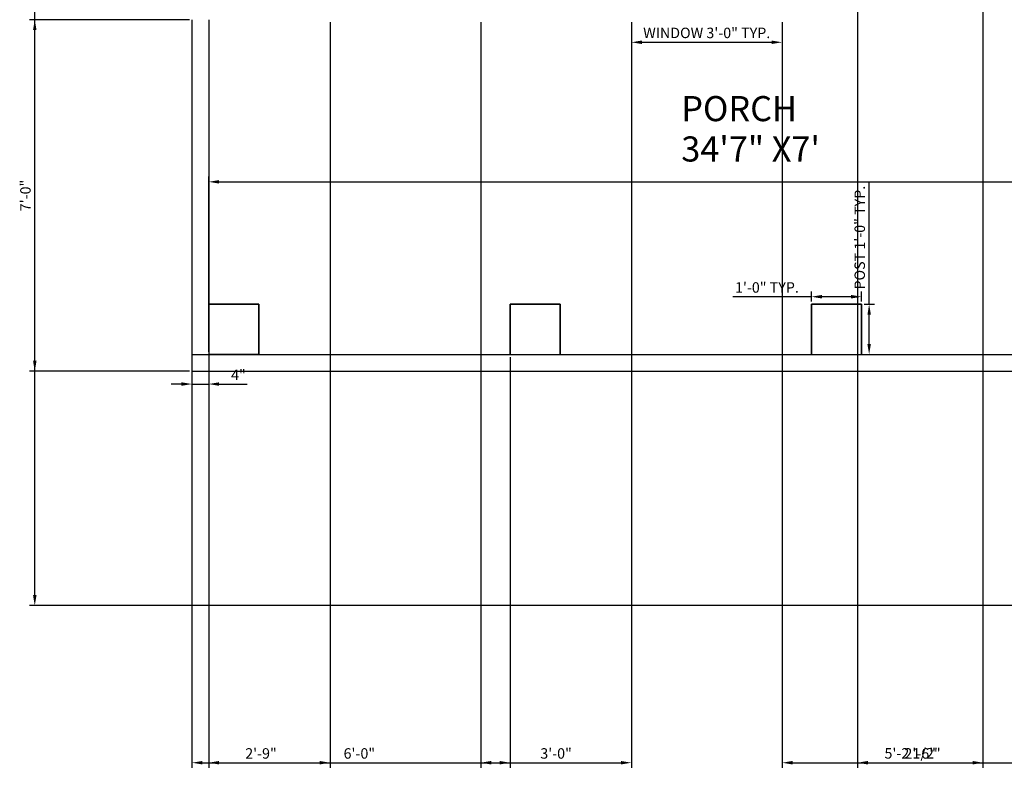
# Model space of a CAD drawing. Units: inches. Extents: x 2025 to 2528, y 1525 to 2336.
# Tile 1 of 18: x 2025 to 2260, y 1525 to 1704. Entities that reach past the tile are written whole.
import ezdxf

# ---------------------------------------------------------------- set-up
doc = ezdxf.new("R2010")
doc.units = ezdxf.units.IN
for name, color, linetype, lineweight in [('A-ANNO-DIMS', 2, 'Continuous', 18), ('A-AREA-IDEN', 7, 'Continuous', 25), ('A-COLS', 7, 'Continuous', 35), ('A-FLOR', 7, 'Continuous', 25)]:
    doc.layers.add(name, color=color, linetype=linetype, lineweight=lineweight)
doc.styles.get("Standard").update_dxf_attribs({"font": 'arial.ttf'})
doc.dimstyles.new('Copy of ISO-25', dxfattribs={"dimtxt": 2.5, "dimasz": 2.5, "dimexe": 1.25, "dimexo": 0.625, "dimtad": 1, "dimdec": 1, "dimlunit": 4, "dimtxsty": 'Standard', "dimcen": 2.5, "dimadec": 0, "dimazin": 0, "dimtfac": 1, "dimtdec": 1, "dimtmove": 0, "dimatfit": 3, "dimfxl": 1, "dimarcsym": 0})

# ---------------------------------------------------------------- blocks, each defined once
blk = doc.blocks.new('*D40')
at = {"layer": 'A-ANNO-DIMS', "color": 0, "lineweight": -2, "transparency": 16777216}
for p, q in [((2070.01, 1625.04), (2070.01, 1666.92)), ((2072.51, 1665.67), (2482.51, 1665.67)), ((2485.01, 1625.04), (2485.01, 1666.92))]:
    blk.add_line(p, q, dxfattribs=at)
at = {"layer": 'A-ANNO-DIMS', "color": 0, "transparency": 16777216}
for points in [[(2072.51, 1666.08), (2072.51, 1665.25), (2070.01, 1665.67)], [(2482.51, 1666.08), (2482.51, 1665.25), (2485.01, 1665.67)]]:
    blk.add_solid(points, dxfattribs=at)
at = {"layer": 'Defpoints', "color": 0, "transparency": 16777216}
for p in [(2485.01, 1665.67), (2070.01, 1624.41), (2485.01, 1624.41)]:
    blk.add_point(p, dxfattribs=at)
at = {"layer": 'A-ANNO-DIMS', "color": 0, "transparency": 16777216, "insert": (2277.51, 1667.57), "char_height": 2.5, "attachment_point": 5}
blk.add_mtext('34\'-7"', dxfattribs=at)
blk = doc.blocks.new('*D44')
at = {"layer": 'A-ANNO-DIMS', "color": 0, "lineweight": -2, "transparency": 16777216}
for p, q in [((2066.01, 1619.79), (2066.01, 1616.1)), ((2070.01, 1619.79), (2070.01, 1616.1)), ((2063.51, 1617.35), (2061.01, 1617.35)), ((2066.01, 1617.35), (2070.01, 1617.35)), ((2072.51, 1617.35), (2079.24, 1617.35))]:
    blk.add_line(p, q, dxfattribs=at)
at = {"layer": 'A-ANNO-DIMS', "color": 0, "transparency": 16777216}
for points in [[(2063.51, 1617.76), (2063.51, 1616.93), (2066.01, 1617.35)], [(2072.51, 1617.76), (2072.51, 1616.93), (2070.01, 1617.35)]]:
    blk.add_solid(points, dxfattribs=at)
at = {"layer": 'Defpoints', "color": 0, "transparency": 16777216}
for p in [(2066.01, 1620.41), (2070.01, 1620.41), (2070.01, 1617.35)]:
    blk.add_point(p, dxfattribs=at)
at = {"layer": 'A-ANNO-DIMS', "color": 0, "transparency": 16777216, "insert": (2077.12, 1619.22), "char_height": 2.5, "attachment_point": 5}
blk.add_mtext('4"', dxfattribs=at)
blk = doc.blocks.new('POST-PORCH-12')
for p, q in [((12, 12), (0, 12)), ((12, 0), (12, 12)), ((0, 0), (12, 0))]:
    blk.add_line(p, q)
blk = doc.blocks.new('*D50')
at = {"layer": 'A-ANNO-DIMS', "color": 0, "lineweight": -2, "transparency": 16777216}
for p, q in [((2227.81, 1636.41), (2227.81, 1665.76)), ((2226.64, 1636.41), (2229.06, 1636.41)), ((2227.81, 1626.91), (2227.81, 1633.91)), ((2226.64, 1624.41), (2229.06, 1624.41))]:
    blk.add_line(p, q, dxfattribs=at)
at = {"layer": 'A-ANNO-DIMS', "color": 0, "transparency": 16777216}
for points in [[(2227.4, 1633.91), (2228.23, 1633.91), (2227.81, 1636.41)], [(2227.4, 1626.91), (2228.23, 1626.91), (2227.81, 1624.41)]]:
    blk.add_solid(points, dxfattribs=at)
at = {"layer": 'Defpoints', "color": 0, "transparency": 16777216}
for p in [(2226.01, 1636.41), (2227.81, 1636.41), (2226.01, 1624.41)]:
    blk.add_point(p, dxfattribs=at)
at = {"layer": 'A-ANNO-DIMS', "color": 0, "transparency": 16777216, "insert": (2225.89, 1652.33), "char_height": 2.5, "attachment_point": 5, "rotation": 90}
blk.add_mtext('POST 1\'-0" TYP.', dxfattribs=at)
blk = doc.blocks.new('*D51')
at = {"layer": 'A-ANNO-DIMS', "color": 0, "lineweight": -2, "transparency": 16777216}
for p, q in [((2214.01, 1638.21), (2195.26, 1638.21)), ((2214.01, 1637.04), (2214.01, 1639.46)), ((2223.51, 1638.21), (2216.51, 1638.21)), ((2226.01, 1637.04), (2226.01, 1639.46))]:
    blk.add_line(p, q, dxfattribs=at)
at = {"layer": 'A-ANNO-DIMS', "color": 0, "transparency": 16777216}
for points in [[(2216.51, 1638.63), (2216.51, 1637.8), (2214.01, 1638.21)], [(2223.51, 1638.63), (2223.51, 1637.8), (2226.01, 1638.21)]]:
    blk.add_solid(points, dxfattribs=at)
at = {"layer": 'Defpoints', "color": 0, "transparency": 16777216}
for p in [(2214.01, 1638.21), (2214.01, 1636.41), (2226.01, 1636.41)]:
    blk.add_point(p, dxfattribs=at)
at = {"layer": 'A-ANNO-DIMS', "color": 0, "transparency": 16777216, "insert": (2203.39, 1640.11), "char_height": 2.5, "attachment_point": 5}
blk.add_mtext('1\'-0" TYP.', dxfattribs=at)
blk = doc.blocks.new('*D52')
at = {"layer": 'A-ANNO-DIMS', "color": 0, "lineweight": -2, "transparency": 16777216}
for p, q in [((2171.01, 1703.79), (2171.01, 1697.76)), ((2207.01, 1703.79), (2207.01, 1697.76)), ((2173.51, 1699.01), (2204.51, 1699.01))]:
    blk.add_line(p, q, dxfattribs=at)
at = {"layer": 'A-ANNO-DIMS', "color": 0, "transparency": 16777216}
for points in [[(2173.51, 1699.43), (2173.51, 1698.6), (2171.01, 1699.01)], [(2204.51, 1699.43), (2204.51, 1698.6), (2207.01, 1699.01)]]:
    blk.add_solid(points, dxfattribs=at)
at = {"layer": 'Defpoints', "color": 0, "transparency": 16777216}
for p in [(2171.01, 1704.41), (2207.01, 1704.41), (2207.01, 1699.01)]:
    blk.add_point(p, dxfattribs=at)
at = {"layer": 'A-ANNO-DIMS', "color": 0, "transparency": 16777216, "insert": (2189.01, 1700.93), "char_height": 2.5, "attachment_point": 5}
blk.add_mtext('WINDOW 3\'-0" TYP.', dxfattribs=at)
blk = doc.blocks.new('*D65')
at = {"layer": 'A-ANNO-DIMS', "color": 0, "lineweight": -2, "transparency": 16777216}
for p, q in [((2066.01, 1703.79), (2066.01, 1525.61)), ((2099.01, 1703.79), (2099.01, 1525.61)), ((2068.51, 1526.86), (2096.51, 1526.86))]:
    blk.add_line(p, q, dxfattribs=at)
at = {"layer": 'A-ANNO-DIMS', "color": 0, "transparency": 16777216}
for points in [[(2068.51, 1527.28), (2068.51, 1526.45), (2066.01, 1526.86)], [(2096.51, 1527.28), (2096.51, 1526.45), (2099.01, 1526.86)]]:
    blk.add_solid(points, dxfattribs=at)
at = {"layer": 'Defpoints', "color": 0, "transparency": 16777216}
for p in [(2066.01, 1704.41), (2099.01, 1704.41), (2099.01, 1526.86)]:
    blk.add_point(p, dxfattribs=at)
at = {"layer": 'A-ANNO-DIMS', "color": 0, "transparency": 16777216, "insert": (2082.51, 1528.76), "char_height": 2.5, "attachment_point": 5}
blk.add_mtext('2\'-9"', dxfattribs=at)
blk = doc.blocks.new('*D66')
at = {"layer": 'A-ANNO-DIMS', "color": 0, "lineweight": -2, "transparency": 16777216}
for p, q in [((2135.01, 1703.79), (2135.01, 1525.61)), ((2171.01, 1703.79), (2171.01, 1525.61)), ((2137.51, 1526.86), (2168.51, 1526.86))]:
    blk.add_line(p, q, dxfattribs=at)
at = {"layer": 'A-ANNO-DIMS', "color": 0, "transparency": 16777216}
for points in [[(2137.51, 1527.28), (2137.51, 1526.45), (2135.01, 1526.86)], [(2168.51, 1527.28), (2168.51, 1526.45), (2171.01, 1526.86)]]:
    blk.add_solid(points, dxfattribs=at)
at = {"layer": 'Defpoints', "color": 0, "transparency": 16777216}
for p in [(2135.01, 1704.41), (2171.01, 1704.41), (2171.01, 1526.86)]:
    blk.add_point(p, dxfattribs=at)
at = {"layer": 'A-ANNO-DIMS', "color": 0, "transparency": 16777216, "insert": (2153.01, 1528.76), "char_height": 2.5, "attachment_point": 5}
blk.add_mtext('3\'-0"', dxfattribs=at)
blk = doc.blocks.new('*D67')
at = {"layer": 'A-ANNO-DIMS', "color": 0, "lineweight": -2, "transparency": 16777216}
for p, q in [((2207.01, 1703.79), (2207.01, 1525.61)), ((2269.37, 1703.79), (2269.37, 1525.61)), ((2209.51, 1526.86), (2266.87, 1526.86))]:
    blk.add_line(p, q, dxfattribs=at)
at = {"layer": 'A-ANNO-DIMS', "color": 0, "transparency": 16777216}
for points in [[(2209.51, 1527.28), (2209.51, 1526.45), (2207.01, 1526.86)], [(2266.87, 1527.28), (2266.87, 1526.45), (2269.37, 1526.86)]]:
    blk.add_solid(points, dxfattribs=at)
at = {"layer": 'Defpoints', "color": 0, "transparency": 16777216}
for p in [(2207.01, 1704.41), (2269.37, 1704.41), (2269.37, 1526.86)]:
    blk.add_point(p, dxfattribs=at)
at = {"layer": 'A-ANNO-DIMS', "color": 0, "transparency": 16777216, "insert": (2238.19, 1528.78), "char_height": 2.5, "attachment_point": 5}
blk.add_mtext('5\'-2 1/2"', dxfattribs=at)
blk = doc.blocks.new('*D70')
at = {"layer": 'A-ANNO-DIMS', "color": 0, "lineweight": -2, "transparency": 16777216}
for p, q in [((2070.01, 1623.79), (2070.01, 1525.61)), ((2142.01, 1623.79), (2142.01, 1525.61)), ((2072.51, 1526.86), (2139.51, 1526.86))]:
    blk.add_line(p, q, dxfattribs=at)
at = {"layer": 'A-ANNO-DIMS', "color": 0, "transparency": 16777216}
for points in [[(2072.51, 1527.28), (2072.51, 1526.45), (2070.01, 1526.86)], [(2139.51, 1527.28), (2139.51, 1526.45), (2142.01, 1526.86)]]:
    blk.add_solid(points, dxfattribs=at)
at = {"layer": 'Defpoints', "color": 0, "transparency": 16777216}
for p in [(2070.01, 1624.41), (2142.01, 1624.41), (2142.01, 1526.86)]:
    blk.add_point(p, dxfattribs=at)
at = {"layer": 'A-ANNO-DIMS', "color": 0, "transparency": 16777216, "insert": (2106.01, 1528.76), "char_height": 2.5, "attachment_point": 5}
blk.add_mtext('6\'-0"', dxfattribs=at)
blk = doc.blocks.new('*D73')
at = {"layer": 'A-ANNO-DIMS', "color": 0, "lineweight": -2, "transparency": 16777216}
for p, q in [((2065.39, 1704.41), (2027.21, 1704.41)), ((2028.46, 1622.91), (2028.46, 1701.91)), ((2065.39, 1620.41), (2027.21, 1620.41))]:
    blk.add_line(p, q, dxfattribs=at)
at = {"layer": 'A-ANNO-DIMS', "color": 0, "transparency": 16777216}
for points in [[(2028.05, 1701.91), (2028.88, 1701.91), (2028.46, 1704.41)], [(2028.05, 1622.91), (2028.88, 1622.91), (2028.46, 1620.41)]]:
    blk.add_solid(points, dxfattribs=at)
at = {"layer": 'Defpoints', "color": 0, "transparency": 16777216}
for p in [(2028.46, 1704.41), (2066.01, 1704.41), (2066.01, 1620.41)]:
    blk.add_point(p, dxfattribs=at)
at = {"layer": 'A-ANNO-DIMS', "color": 0, "transparency": 16777216, "insert": (2026.56, 1662.41), "char_height": 2.5, "attachment_point": 5, "rotation": 90}
blk.add_mtext('7\'-0"', dxfattribs=at)
blk = doc.blocks.new('*D75')
at = {"layer": 'A-ANNO-DIMS', "color": 0, "lineweight": -2, "transparency": 16777216}
for p, q in [((2225.01, 2114.79), (2225.01, 1525.61)), ((2255.01, 2114.79), (2255.01, 1525.61)), ((2227.51, 1526.86), (2252.51, 1526.86))]:
    blk.add_line(p, q, dxfattribs=at)
at = {"layer": 'A-ANNO-DIMS', "color": 0, "transparency": 16777216}
for points in [[(2227.51, 1527.28), (2227.51, 1526.45), (2225.01, 1526.86)], [(2252.51, 1527.28), (2252.51, 1526.45), (2255.01, 1526.86)]]:
    blk.add_solid(points, dxfattribs=at)
at = {"layer": 'Defpoints', "color": 0, "transparency": 16777216}
for p in [(2225.01, 2115.41), (2255.01, 2115.41), (2255.01, 1526.86)]:
    blk.add_point(p, dxfattribs=at)
at = {"layer": 'A-ANNO-DIMS', "color": 0, "transparency": 16777216, "insert": (2240.01, 1528.76), "char_height": 2.5, "attachment_point": 5}
blk.add_mtext('2\'-6"', dxfattribs=at)
blk = doc.blocks.new('*D80')
at = {"layer": 'A-ANNO-DIMS', "color": 0, "lineweight": -2, "transparency": 16777216}
for p, q in [((2065.39, 2292.41), (2027.21, 2292.41)), ((2028.46, 1566.91), (2028.46, 2289.91)), ((2285.39, 1564.41), (2027.21, 1564.41))]:
    blk.add_line(p, q, dxfattribs=at)
at = {"layer": 'A-ANNO-DIMS', "color": 0, "transparency": 16777216}
for points in [[(2028.05, 2289.91), (2028.88, 2289.91), (2028.46, 2292.41)], [(2028.05, 1566.91), (2028.88, 1566.91), (2028.46, 1564.41)]]:
    blk.add_solid(points, dxfattribs=at)
at = {"layer": 'Defpoints', "color": 0, "transparency": 16777216}
for p in [(2028.46, 2292.41), (2066.01, 2292.41), (2286.01, 1564.41)]:
    blk.add_point(p, dxfattribs=at)
at = {"layer": 'A-ANNO-DIMS', "color": 0, "transparency": 16777216, "insert": (2026.56, 1928.41), "char_height": 2.5, "attachment_point": 5, "rotation": 90}
blk.add_mtext('60\'-8"', dxfattribs=at)

msp = doc.modelspace()

# ---------------------------------------------------------------- linework, layer by layer
at = {"layer": 'A-FLOR'}
for p, q in [((2066.01, 1704.41), (2066.01, 1620.41)), ((2070.01, 1704.41), (2070.01, 1620.41)), ((2066.01, 1624.41), (2489.01, 1624.41)), ((2082.01, 1624.41), (2142.01, 1624.41)), ((2154.01, 1624.41), (2214.01, 1624.41)), ((2226.01, 1624.41), (2286.01, 1624.41)), ((2066.01, 1620.41), (2489.01, 1620.41))]:
    msp.add_line(p, q, dxfattribs=at)

# ---------------------------------------------------------------- block references
at = {"layer": 'A-COLS'}
msp.add_blockref('POST-PORCH-12', (2070.01, 1624.41), dxfattribs=at)
at = {"layer": 'A-COLS', "rotation": 90}
for p in [(2154.01, 1624.41), (2226.01, 1624.41)]:
    msp.add_blockref('POST-PORCH-12', p, dxfattribs=at)

# ---------------------------------------------------------------- texts
at = {"layer": 'A-AREA-IDEN'}
for s, p in [('PORCH', (2182.93, 1680.16)), ('34\'7" X7\'', (2182.93, 1670.52))]:
    msp.add_text(s, height=6, dxfattribs=at).set_placement(p)

# ---------------------------------------------------------------- dimensions: what is measured, and where the dimension line sits
at = {"layer": 'A-ANNO-DIMS'}
for base, p1, p2, picture, middle in [((2028.46, 2292.41), (2286.01, 1564.41), (2066.01, 2292.41), '*D80', (2026.56, 1928.41)), ((2028.46, 1704.41), (2066.01, 1620.41), (2066.01, 1704.41), '*D73', (2026.56, 1662.41))]:
    dim = msp.add_linear_dim(base=base, p1=p1, p2=p2, angle=90, dimstyle='Copy of ISO-25', override={"dimdec": 1, "dimlfac": 1, "dimrnd": 0, "dimzin": 1, "dimdsep": 46, "dimlunit": 4, "dimfrac": 2}, dxfattribs=at)
    dim.commit()
    dim.dimension.update_dxf_attribs({"geometry": picture, "text_midpoint": middle})
for base, p1, p2, override, picture, middle in [((2255.01, 1526.86), (2225.01, 2115.41), (2255.01, 2115.41), {"dimdec": 1, "dimlfac": 1, "dimrnd": 0, "dimzin": 1, "dimdsep": 46, "dimlunit": 4, "dimfrac": 2}, '*D75', (2240.01, 1528.76)), ((2099.01, 1526.86), (2066.01, 1704.41), (2099.01, 1704.41), {"dimdec": 1, "dimlfac": 1, "dimrnd": 0, "dimzin": 1, "dimdsep": 46, "dimlunit": 4, "dimfrac": 2}, '*D65', (2082.51, 1528.76)), ((2171.01, 1526.86), (2135.01, 1704.41), (2171.01, 1704.41), {"dimdec": 1, "dimlfac": 1, "dimrnd": 0, "dimzin": 1, "dimdsep": 46, "dimlunit": 4, "dimfrac": 2}, '*D66', (2153.01, 1528.76)), ((2269.37, 1526.86), (2207.01, 1704.41), (2269.37, 1704.41), {"dimdec": 1, "dimlfac": 1, "dimrnd": 0, "dimzin": 1, "dimdsep": 46, "dimlunit": 4, "dimfrac": 2}, '*D67', (2238.19, 1528.78)), ((2485.01, 1665.67), (2070.01, 1624.41), (2485.01, 1624.41), {"dimclrd": 0, "dimclre": 0, "dimclrt": 0}, '*D40', (2277.51, 1667.57)), ((2142.01, 1526.86), (2070.01, 1624.41), (2142.01, 1624.41), {"dimdec": 1, "dimlfac": 1, "dimrnd": 0, "dimzin": 1, "dimdsep": 46, "dimlunit": 4, "dimfrac": 2}, '*D70', (2106.01, 1528.76)), ((2070.01, 1617.35), (2066.01, 1620.41), (2070.01, 1620.41), {"dimclrd": 0, "dimclre": 0, "dimclrt": 0}, '*D44', (2077.12, 1619.22))]:
    dim = msp.add_linear_dim(base=base, p1=p1, p2=p2, dimstyle='Copy of ISO-25', override=override, dxfattribs=at)
    dim.commit()
    dim.dimension.update_dxf_attribs({"geometry": picture, "text_midpoint": middle})
dim = msp.add_linear_dim(base=(2207.01, 1699.01), p1=(2171.01, 1704.41), p2=(2207.01, 1704.41), text='WINDOW <> TYP.', dimstyle='Copy of ISO-25', override={"dimdec": 1, "dimlfac": 1, "dimrnd": 0, "dimzin": 1, "dimdsep": 46, "dimlunit": 4, "dimfrac": 2}, dxfattribs=at)
dim.commit()
dim.dimension.update_dxf_attribs({"geometry": '*D52', "text_midpoint": (2189.01, 1700.93)})
for base, p1, p2, angle, text, picture, middle in [((2227.81, 1636.41), (2226.01, 1624.41), (2226.01, 1636.41), 90, 'POST <> TYP.', '*D50', (2225.89, 1652.33)), ((2214.01, 1638.21), (2226.01, 1636.41), (2214.01, 1636.41), 180, '<> TYP.', '*D51', (2203.39, 1640.11))]:
    dim = msp.add_linear_dim(base=base, p1=p1, p2=p2, angle=angle, text=text, dimstyle='Copy of ISO-25', override={"dimdec": 1, "dimlfac": 1, "dimrnd": 0, "dimzin": 1, "dimdsep": 46, "dimlunit": 4, "dimfrac": 2}, dxfattribs=at)
    dim.commit()
    dim.dimension.update_dxf_attribs({"geometry": picture, "text_midpoint": middle})

doc.saveas('drawing.dxf')
